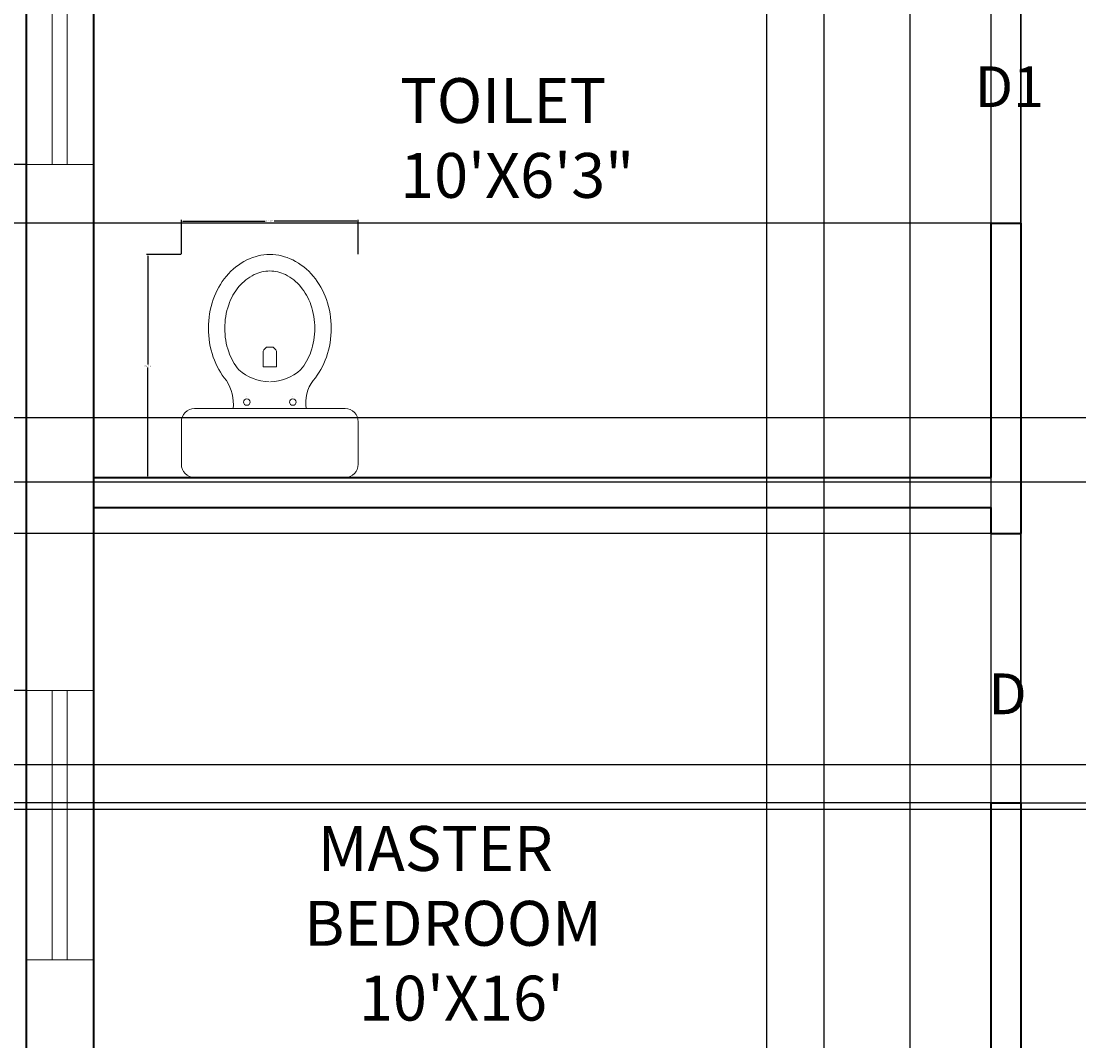
# Model space of a CAD drawing. Units: inches. Extents: x 503 to 1084, y -605 to 132.
# Tile 5 of 14: x 649 to 791, y -313 to -177. Entities that reach past the tile are written whole.
import ezdxf

# ---------------------------------------------------------------- set-up
doc = ezdxf.new("R2010")
doc.units = ezdxf.units.IN
doc.header["$MEASUREMENT"] = 0
for name, color, linetype, lineweight in [('A-ANNO-DIMS', 7, 'Continuous', 18), ('A-ANNO-TEXT', 7, 'Continuous', 18), ('A-AREA-IDEN', 8, 'Continuous', 18), ('A-FLOR-FIXT', 8, 'Continuous', 18), ('wall', 1, 'Continuous', 35), ('wind', 5, 'Continuous', 18)]:
    doc.layers.add(name, color=color, linetype=linetype, lineweight=lineweight)
doc.styles.get("Standard").update_dxf_attribs({"font": 'arial.ttf'})
doc.dimstyles.get("Standard").update_dxf_attribs({"dimtxt": 0.18, "dimasz": 0.18, "dimexe": 0.18, "dimexo": 0.0625, "dimgap": 0.09, "dimtad": 0, "dimtih": 1, "dimtoh": 1, "dimdec": 1, "dimzin": 0, "dimdsep": 46, "dimlunit": 4, "dimtxsty": 'Standard', "dimcen": 0.09, "dimadec": 0, "dimazin": 0, "dimtfac": 1, "dimtdec": 1, "dimtofl": 0, "dimtmove": 0, "dimatfit": 3, "dimfxl": 1, "dimtolj": 1, "dimtzin": 0, "dimarcsym": 0})

# ---------------------------------------------------------------- blocks, each defined once
blk = doc.blocks.new('WC-P01')
for p, q in [((-230, 0), (230, 0)), ((-270, -40), (-270, -170)), ((270, -40), (270, -170)), ((-230, -210), (230, -210)), ((-111.4, -210), (-111.4, -210)), ((-20, -337.8), (20, -337.8)), ((-20, -337.8), (-20, -385.7)), ((20, -337.8), (20, -385.7)), ((-18.5, -389.3), (-10.5, -397.3)), ((-10.5, -397.3), (10.5, -397.3)), ((10.5, -397.3), (18.5, -389.3))]:
    blk.add_line(p, q)
for points in [[(-111.4, -210, -0.215497), (-132.6, -295.9, 0.09084), (-172.8, -367.1, 0.083285), (-187.5, -455, 0.083285), (-172.8, -542.9, 0.09084), (-132.6, -614.1, 0.104065), (-70, -663.6, 0.115836), (0, -680, 0.115836), (70, -663.6, 0.104065), (132.6, -614.1, 0.09084), (172.8, -542.9, 0.083285), (187.5, -455, 0.083285)], [(187.5, -455, 0.083285), (172.8, -367.1, 0.09084), (132.6, -295.9, -0.156524), (111.4, -210)], [(-70, -246.4), (-70, -246.4, 0.104065)], [(70, -246.4), (70, -246.4, 0.115836)], [(-1.8, -291.3, 0.171753), (-94.2, -327.9, 0.09084), (-125.5, -383.5, 0.083285), (-137.5, -455, 0.083285), (-125.5, -526.5, 0.09084), (-94.2, -582.1, 0.104065), (-47.7, -618.8, 0.115836), (0, -630, 0.115836)], [(1.8, -291.3, -0.171753), (94.2, -327.9, -0.09084), (125.5, -383.5, -0.083285), (137.5, -455, -0.083285), (125.5, -526.5, -0.09084), (94.2, -582.1, -0.104065), (47.7, -618.8, -0.115836), (0, -630, -0.115836)]]:
    blk.add_lwpolyline(points, format="xyb")
for centre in [(-70, -230), (70, -230)]:
    blk.add_circle(centre, 10)
for centre, radius, start, end in [((-230, -40), 40, 90, 180), ((230, -40), 40, 0, 90), ((-230, -170), 40, 180, 270), ((230, -170), 40, 270, 0), ((-15, -385.7), 5, 180, 225), ((15, -385.7), 5, 315, 0)]:
    blk.add_arc(centre, radius, start, end)
blk = doc.blocks.new('_ArchTick')
at = {"color": 0, "linetype": 'ByBlock', "const_width": 0.15}
blk.add_lwpolyline([(-0.5, -0.5), (0.5, 0.5)], dxfattribs=at)
blk = doc.blocks.new('_Oblique')
at = {"color": 0, "linetype": 'ByBlock', "lineweight": -2}
blk.add_line((-0.5, -0.5), (0.5, 0.5), dxfattribs=at)
blk = doc.blocks.new('*D12')
at = {"layer": 'A-ANNO-DIMS', "color": 0, "lineweight": -2, "transparency": 16777216}
blk.add_line((554.79, -17.82), (554.79, -442.82), dxfattribs=at)
at = {"layer": 'Defpoints', "color": 0, "transparency": 16777216}
for p in [(650.09, -17.82), (554.79, -442.82), (650.09, -442.82)]:
    blk.add_point(p, dxfattribs=at)
at = {"layer": 'A-ANNO-DIMS', "color": 0, "lineweight": -2, "transparency": 16777216, "xscale": 5, "yscale": 5, "zscale": 5}
for name, p, rotation in [('_ArchTick', (554.79, -17.82), 90), ('_Oblique', (554.79, -442.82), 270)]:
    blk.add_blockref(name, p, dxfattribs=dict(at, rotation=rotation))
at = {"layer": 'A-ANNO-DIMS', "color": 0, "transparency": 16777216, "insert": (546.7, -230.32), "char_height": 8, "attachment_point": 5, "rotation": 90}
blk.add_mtext("\\A1;36'", dxfattribs=at)
blk = doc.blocks.new('WIN-36IN')
for p, q in [((0, 0), (0, 9)), ((36, 0), (36, 9)), ((0, 5.5), (36, 5.5)), ((0, 3.5), (36, 3.5))]:
    blk.add_line(p, q)
blk = doc.blocks.new('VENT-24IN')
for p, q in [((0, 9), (0, 0)), ((24, 9), (24, 0)), ((24, 5.5), (0, 5.5)), ((24, 3.5), (0, 3.5))]:
    blk.add_line(p, q)
blk = doc.blocks.new('*D32')
at = {"layer": 'A-ANNO-DIMS', "color": 0, "lineweight": -2, "transparency": 16777216}
for p, q in [((670.79, -208.03), (666.21, -208.03)), ((666.39, -208.21), (666.39, -222.74)), ((666.39, -237.64), (666.39, -223.11)), ((670.79, -237.82), (666.21, -237.82))]:
    blk.add_line(p, q, dxfattribs=at)
at = {"layer": 'A-ANNO-DIMS', "color": 0, "transparency": 16777216}
for points in [[(666.36, -208.21), (666.42, -208.21), (666.39, -208.03)], [(666.36, -237.64), (666.42, -237.64), (666.39, -237.82)]]:
    blk.add_solid(points, dxfattribs=at)
at = {"layer": 'Defpoints', "color": 0, "transparency": 16777216}
for p in [(670.86, -208.03), (666.39, -237.82), (670.86, -237.82)]:
    blk.add_point(p, dxfattribs=at)
at = {"layer": 'A-ANNO-DIMS', "color": 0, "transparency": 16777216, "insert": (666.39, -222.92), "char_height": 0.18, "attachment_point": 5}
blk.add_mtext('\\A1;WC 2\'-6"', dxfattribs=at)
blk = doc.blocks.new('*D33')
at = {"layer": 'A-ANNO-DIMS', "color": 0, "lineweight": -2, "transparency": 16777216}
for p, q in [((670.86, -207.97), (670.86, -203.38)), ((671.04, -203.56), (682.08, -203.56)), ((694.33, -203.56), (683.28, -203.56)), ((694.51, -207.97), (694.51, -203.38))]:
    blk.add_line(p, q, dxfattribs=at)
at = {"layer": 'A-ANNO-DIMS', "color": 0, "transparency": 16777216}
for points in [[(671.04, -203.53), (671.04, -203.59), (670.86, -203.56)], [(694.33, -203.53), (694.33, -203.59), (694.51, -203.56)]]:
    blk.add_solid(points, dxfattribs=at)
at = {"layer": 'Defpoints', "color": 0, "transparency": 16777216}
for p in [(670.86, -203.56), (670.86, -208.03), (694.51, -208.03)]:
    blk.add_point(p, dxfattribs=at)
at = {"layer": 'A-ANNO-DIMS', "color": 0, "transparency": 16777216, "insert": (682.68, -203.56), "char_height": 0.18, "attachment_point": 5}
blk.add_mtext('\\A1;1\'-11 1/2"', dxfattribs=at)
blk = doc.blocks.new('*D48')
at = {"layer": 'A-ANNO-DIMS', "color": 0, "lineweight": -2, "transparency": 16777216}
for p, q in [((783.09, -354.75), (783.09, 43.51)), ((783.27, 43.33), (789.22, 43.33)), ((795.82, 43.33), (789.86, 43.33)), ((796, -354.75), (796, 43.51))]:
    blk.add_line(p, q, dxfattribs=at)
at = {"layer": 'A-ANNO-DIMS', "color": 0, "transparency": 16777216}
for points in [[(783.27, 43.36), (783.27, 43.3), (783.09, 43.33)], [(795.82, 43.36), (795.82, 43.3), (796, 43.33)]]:
    blk.add_solid(points, dxfattribs=at)
at = {"layer": 'Defpoints', "color": 0, "transparency": 16777216}
for p in [(796, 43.33), (783.09, -354.82), (796, -354.82)]:
    blk.add_point(p, dxfattribs=at)
at = {"layer": 'A-ANNO-DIMS', "color": 0, "transparency": 16777216, "insert": (789.54, 43.33), "char_height": 0.18, "attachment_point": 5}
blk.add_mtext('\\A1;1\'-1"', dxfattribs=at)
blk = doc.blocks.new('*D54')
at = {"layer": 'A-ANNO-DIMS', "color": 0, "lineweight": -2, "transparency": 16777216}
for p, q in [((650.03, -195.98), (552.76, -195.98)), ((552.94, -196.16), (552.94, -230.97)), ((552.94, -266.14), (552.94, -231.33)), ((650.03, -266.32), (552.76, -266.32))]:
    blk.add_line(p, q, dxfattribs=at)
at = {"layer": 'A-ANNO-DIMS', "color": 0, "transparency": 16777216}
for points in [[(552.91, -196.16), (552.97, -196.16), (552.94, -195.98)], [(552.91, -266.14), (552.97, -266.14), (552.94, -266.32)]]:
    blk.add_solid(points, dxfattribs=at)
at = {"layer": 'Defpoints', "color": 0, "transparency": 16777216}
for p in [(650.09, -195.98), (552.94, -266.32), (650.09, -266.32)]:
    blk.add_point(p, dxfattribs=at)
at = {"layer": 'A-ANNO-DIMS', "color": 0, "transparency": 16777216, "insert": (552.94, -231.15), "char_height": 0.18, "attachment_point": 5}
blk.add_mtext('\\A1;5\'-10 1/2"', dxfattribs=at)
blk = doc.blocks.new('*D55')
at = {"layer": 'A-ANNO-DIMS', "color": 0, "lineweight": -2, "transparency": 16777216}
for p, q in [((779.03, -245.32), (552.76, -245.32)), ((552.94, -245.5), (552.94, -263.13)), ((552.94, -281.14), (552.94, -263.5)), ((779.03, -281.32), (552.76, -281.32))]:
    blk.add_line(p, q, dxfattribs=at)
at = {"layer": 'A-ANNO-DIMS', "color": 0, "transparency": 16777216}
for points in [[(552.91, -245.5), (552.97, -245.5), (552.94, -245.32)], [(552.91, -281.14), (552.97, -281.14), (552.94, -281.32)]]:
    blk.add_solid(points, dxfattribs=at)
at = {"layer": 'Defpoints', "color": 0, "transparency": 16777216}
for p in [(779.09, -245.32), (552.94, -281.32), (779.09, -281.32)]:
    blk.add_point(p, dxfattribs=at)
at = {"layer": 'A-ANNO-DIMS', "color": 0, "transparency": 16777216, "insert": (552.94, -263.32), "char_height": 0.18, "attachment_point": 5}
blk.add_mtext('\\A1;3\'-0"', dxfattribs=at)
blk = doc.blocks.new('*D56')
at = {"layer": 'A-ANNO-DIMS', "color": 0, "lineweight": -2, "transparency": 16777216}
for p, q in [((779.03, -167.82), (552.76, -167.82)), ((552.94, -168), (552.94, -185.63)), ((552.94, -203.64), (552.94, -186)), ((779.03, -203.82), (552.76, -203.82))]:
    blk.add_line(p, q, dxfattribs=at)
at = {"layer": 'A-ANNO-DIMS', "color": 0, "transparency": 16777216}
for points in [[(552.91, -168), (552.97, -168), (552.94, -167.82)], [(552.91, -203.64), (552.97, -203.64), (552.94, -203.82)]]:
    blk.add_solid(points, dxfattribs=at)
at = {"layer": 'Defpoints', "color": 0, "transparency": 16777216}
for p in [(779.09, -167.82), (552.94, -203.82), (779.09, -203.82)]:
    blk.add_point(p, dxfattribs=at)
at = {"layer": 'A-ANNO-DIMS', "color": 0, "transparency": 16777216, "insert": (552.94, -185.82), "char_height": 0.18, "attachment_point": 5}
blk.add_mtext('\\A1;3\'-0"', dxfattribs=at)
blk = doc.blocks.new('*D60')
at = {"layer": 'A-ANNO-DIMS', "color": 0, "lineweight": -2, "transparency": 16777216}
for p, q in [((749.09, -117.88), (749.09, -583.15)), ((779.09, -117.88), (779.09, -583.15)), ((749.27, -582.97), (763.76, -582.97)), ((778.91, -582.97), (764.42, -582.97))]:
    blk.add_line(p, q, dxfattribs=at)
at = {"layer": 'A-ANNO-DIMS', "color": 0, "transparency": 16777216}
for points in [[(749.27, -582.94), (749.27, -583), (749.09, -582.97)], [(778.91, -582.94), (778.91, -583), (779.09, -582.97)]]:
    blk.add_solid(points, dxfattribs=at)
at = {"layer": 'Defpoints', "color": 0, "transparency": 16777216}
for p in [(749.09, -117.82), (779.09, -117.82), (779.09, -582.97)]:
    blk.add_point(p, dxfattribs=at)
at = {"layer": 'A-ANNO-DIMS', "color": 0, "transparency": 16777216, "insert": (764.09, -582.97), "char_height": 0.18, "attachment_point": 5}
blk.add_mtext('\\A1;2\'-6"', dxfattribs=at)
blk = doc.blocks.new('*D62')
at = {"layer": 'A-ANNO-DIMS', "color": 0, "lineweight": -2, "transparency": 16777216}
for p, q in [((779.03, -203.82), (552.76, -203.82)), ((552.94, -204), (552.94, -224.38)), ((552.94, -245.14), (552.94, -224.75)), ((779.03, -245.32), (552.76, -245.32))]:
    blk.add_line(p, q, dxfattribs=at)
at = {"layer": 'A-ANNO-DIMS', "color": 0, "transparency": 16777216}
for points in [[(552.91, -204), (552.97, -204), (552.94, -203.82)], [(552.91, -245.14), (552.97, -245.14), (552.94, -245.32)]]:
    blk.add_solid(points, dxfattribs=at)
at = {"layer": 'Defpoints', "color": 0, "transparency": 16777216}
for p in [(779.09, -203.82), (552.94, -245.32), (779.09, -245.32)]:
    blk.add_point(p, dxfattribs=at)
at = {"layer": 'A-ANNO-DIMS', "color": 0, "transparency": 16777216, "insert": (552.94, -224.57), "char_height": 0.18, "attachment_point": 5}
blk.add_mtext('\\A1;3\'-5 1/2"', dxfattribs=at)
blk = doc.blocks.new('*D63')
at = {"layer": 'A-ANNO-DIMS', "color": 0, "lineweight": -2, "transparency": 16777216}
for p, q in [((783.15, -281.32), (1083.42, -281.32)), ((1083.24, -281.5), (1083.24, -317.88)), ((1083.24, -354.64), (1083.24, -318.25)), ((783.15, -354.82), (1083.42, -354.82))]:
    blk.add_line(p, q, dxfattribs=at)
at = {"layer": 'A-ANNO-DIMS', "color": 0, "transparency": 16777216}
for points in [[(1083.21, -281.5), (1083.27, -281.5), (1083.24, -281.32)], [(1083.21, -354.64), (1083.27, -354.64), (1083.24, -354.82)]]:
    blk.add_solid(points, dxfattribs=at)
at = {"layer": 'Defpoints', "color": 0, "transparency": 16777216}
for p in [(783.09, -281.32), (783.09, -354.82), (1083.24, -354.82)]:
    blk.add_point(p, dxfattribs=at)
at = {"layer": 'A-ANNO-DIMS', "color": 0, "transparency": 16777216, "insert": (1083.24, -318.07), "char_height": 0.18, "attachment_point": 5}
blk.add_mtext('\\A1;6\'-1 1/2"', dxfattribs=at)
blk = doc.blocks.new('*D68')
at = {"layer": 'A-ANNO-DIMS', "color": 0, "lineweight": -2, "transparency": 16777216}
for p, q in [((779.09, -117.88), (779.09, -583.15)), ((783.09, -117.88), (783.09, -583.15)), ((779.27, -582.97), (780.76, -582.97)), ((782.91, -582.97), (781.42, -582.97))]:
    blk.add_line(p, q, dxfattribs=at)
at = {"layer": 'A-ANNO-DIMS', "color": 0, "transparency": 16777216}
for points in [[(779.27, -582.94), (779.27, -583), (779.09, -582.97)], [(782.91, -582.94), (782.91, -583), (783.09, -582.97)]]:
    blk.add_solid(points, dxfattribs=at)
at = {"layer": 'Defpoints', "color": 0, "transparency": 16777216}
for p in [(779.09, -117.82), (783.09, -117.82), (783.09, -582.97)]:
    blk.add_point(p, dxfattribs=at)
at = {"layer": 'A-ANNO-DIMS', "color": 0, "transparency": 16777216, "insert": (781.09, -582.97), "char_height": 0.18, "attachment_point": 5}
blk.add_mtext('\\A1;0\'-4"', dxfattribs=at)
blk = doc.blocks.new('*D72')
at = {"layer": 'A-ANNO-DIMS', "color": 0, "lineweight": -2, "transparency": 16777216}
for p, q in [((948.89, -229.87), (552.76, -229.87)), ((552.94, -230.05), (552.94, -255.86)), ((552.94, -282.03), (552.94, -256.22)), ((949.25, -282.21), (552.76, -282.21))]:
    blk.add_line(p, q, dxfattribs=at)
at = {"layer": 'A-ANNO-DIMS', "color": 0, "transparency": 16777216}
for points in [[(552.91, -230.05), (552.97, -230.05), (552.94, -229.87)], [(552.91, -282.03), (552.97, -282.03), (552.94, -282.21)]]:
    blk.add_solid(points, dxfattribs=at)
at = {"layer": 'Defpoints', "color": 0, "transparency": 16777216}
for p in [(948.95, -229.87), (552.94, -282.21), (949.31, -282.21)]:
    blk.add_point(p, dxfattribs=at)
at = {"layer": 'A-ANNO-DIMS', "color": 0, "transparency": 16777216, "insert": (552.94, -256.04), "char_height": 0.18, "attachment_point": 5}
blk.add_mtext('\\A1;4\'-4 1/2"', dxfattribs=at)
blk = doc.blocks.new('*D76')
at = {"layer": 'A-ANNO-DIMS', "color": 0, "lineweight": -2, "transparency": 16777216}
for p, q in [((756.77, -45.47), (756.77, -583.15)), ((768.24, -45.47), (768.24, -583.15)), ((756.95, -582.97), (761.9, -582.97)), ((768.06, -582.97), (763.11, -582.97))]:
    blk.add_line(p, q, dxfattribs=at)
at = {"layer": 'A-ANNO-DIMS', "color": 0, "transparency": 16777216}
for points in [[(756.95, -582.94), (756.95, -583), (756.77, -582.97)], [(768.06, -582.94), (768.06, -583), (768.24, -582.97)]]:
    blk.add_solid(points, dxfattribs=at)
at = {"layer": 'Defpoints', "color": 0, "transparency": 16777216}
for p in [(756.77, -45.4), (768.24, -45.4), (768.24, -582.97)]:
    blk.add_point(p, dxfattribs=at)
at = {"layer": 'A-ANNO-DIMS', "color": 0, "transparency": 16777216, "insert": (762.51, -582.97), "char_height": 0.18, "attachment_point": 5}
blk.add_mtext('\\A1;0\'-11 1/2"', dxfattribs=at)
blk = doc.blocks.new('*D77')
at = {"layer": 'A-ANNO-DIMS', "color": 0, "lineweight": -2, "transparency": 16777216}
for p, q in [((926.53, -238.47), (552.76, -238.47)), ((552.94, -238.65), (552.94, -257.17)), ((552.94, -276.07), (552.94, -257.54)), ((916.28, -276.25), (552.76, -276.25))]:
    blk.add_line(p, q, dxfattribs=at)
at = {"layer": 'A-ANNO-DIMS', "color": 0, "transparency": 16777216}
for points in [[(552.91, -238.65), (552.97, -238.65), (552.94, -238.47)], [(552.91, -276.07), (552.97, -276.07), (552.94, -276.25)]]:
    blk.add_solid(points, dxfattribs=at)
at = {"layer": 'Defpoints', "color": 0, "transparency": 16777216}
for p in [(926.59, -238.47), (552.94, -276.25), (916.35, -276.25)]:
    blk.add_point(p, dxfattribs=at)
at = {"layer": 'A-ANNO-DIMS', "color": 0, "transparency": 16777216, "insert": (552.94, -257.36), "char_height": 0.18, "attachment_point": 5}
blk.add_mtext('\\A1;3\'-2"', dxfattribs=at)

msp = doc.modelspace()

# ---------------------------------------------------------------- linework, layer by layer
at = {"layer": 'wall'}
for p, q in [((650.09, -17.82), (650.09, -514.82)), ((659.09, -26.82), (659.09, -433.82)), ((779.09, -203.82), (783.09, -203.82)), ((779.09, -203.82), (779.09, -237.82)), ((783.09, -203.82), (783.09, -245.32)), ((659.09, -237.82), (779.09, -237.82)), ((659.09, -241.82), (779.09, -241.82)), ((779.09, -241.82), (779.09, -245.32)), ((779.09, -245.32), (783.09, -245.32)), ((779.09, -281.32), (783.09, -281.32)), ((779.09, -281.32), (779.09, -433.82)), ((783.09, -281.32), (783.09, -354.82))]:
    msp.add_line(p, q, dxfattribs=at)

# ---------------------------------------------------------------- block references
at = {"layer": 'A-FLOR-FIXT', "xscale": 0.0438047028060103, "yscale": 0.0438047028060103, "zscale": 0.0438047028060103, "rotation": 180}
msp.add_blockref('WC-P01', (682.68, -237.82), dxfattribs=at)
at = {"layer": 'wind'}
for name, p, rotation in [('VENT-24IN', (659.09, -195.98), 90.00000000000081), ('WIN-36IN', (659.09, -302.31), 90.00000000000033)]:
    msp.add_blockref(name, p, dxfattribs=dict(at, rotation=rotation))

# ---------------------------------------------------------------- texts
at = {"layer": 'A-ANNO-TEXT'}
for s, height, p in [('D1', 5.444, (776.95, -188.32)), ('D', 5.44, (778.77, -269.47))]:
    msp.add_text(s, height=height, dxfattribs=at).set_placement(p)
at = {"layer": 'A-AREA-IDEN', "char_height": 6, "attachment_point": 1}
for s, width, insert in [('       TOILET\\P       10\'X6\'3"', 54.3765, (687.27, -184.45)), (" MASTER BEDROOM\\P    10'X16'", 45.6749, (687.27, -284.42))]:
    msp.add_mtext_dynamic_manual_height_columns(s, width=width, gutter_width=1, heights=[0], dxfattribs=dict(at, insert=insert))

# ---------------------------------------------------------------- dimensions: what is measured, and where the dimension line sits
at = {"layer": 'A-ANNO-DIMS'}
for base, p1, p2, picture, middle in [((796, 43.33), (783.09, -354.82), (796, -354.82), '*D48', (789.54, 43.33)), ((768.24, -582.97), (756.77, -45.4), (768.24, -45.4), '*D76', (762.51, -582.97)), ((779.09, -582.97), (749.09, -117.82), (779.09, -117.82), '*D60', (764.09, -582.97)), ((783.09, -582.97), (779.09, -117.82), (783.09, -117.82), '*D68', (781.09, -582.97))]:
    dim = msp.add_linear_dim(base=base, p1=p1, p2=p2, dimstyle='Standard', override={"dimdec": 1, "dimlfac": 1, "dimrnd": 0, "dimzin": 1, "dimdsep": 46, "dimlunit": 4, "dimfrac": 2}, dxfattribs=at)
    dim.commit()
    dim.dimension.update_dxf_attribs({"geometry": picture, "text_midpoint": middle})
for base, p1, p2, angle, text, override, picture, middle in [((554.79, -442.82), (650.09, -17.82), (650.09, -442.82), 90, "36'", {"dimtxt": 8, "dimasz": 5, "dimgap": 4, "dimtad": 1, "dimtih": 0, "dimblk1": 'ArchTick', "dimblk2": 'Oblique', "dimsah": 1, "dimse1": 1, "dimse2": 1, "dimclrd": 0, "dimclre": 0, "dimclrt": 0}, '*D12', (546.7, -230.32)), ((666.39, -237.82), (670.86, -208.03), (670.86, -237.82), 270, 'WC <>', {"dimdec": 1, "dimlfac": 1, "dimrnd": 0, "dimzin": 1, "dimdsep": 46, "dimlunit": 4, "dimfrac": 2}, '*D32', (666.39, -222.92))]:
    dim = msp.add_linear_dim(base=base, p1=p1, p2=p2, angle=angle, text=text, dimstyle='Standard', override=override, dxfattribs=at)
    dim.commit()
    dim.dimension.update_dxf_attribs({"geometry": picture, "text_midpoint": middle})
for base, p1, p2, angle, picture, middle in [((552.94, -203.82), (779.09, -167.82), (779.09, -203.82), 90, '*D56', (552.94, -185.82)), ((552.94, -266.32), (650.09, -195.98), (650.09, -266.32), 90, '*D54', (552.94, -231.15)), ((670.8553, -203.5606), (694.5099, -208.0287), (670.8553, -208.0287), 180, '*D33', (682.6826, -203.5606)), ((552.94, -245.32), (779.09, -203.82), (779.09, -245.32), 90, '*D62', (552.94, -224.57)), ((552.94, -282.21), (948.95, -229.87), (949.31, -282.21), 90, '*D72', (552.94, -256.04)), ((552.94, -276.25), (926.59, -238.47), (916.35, -276.25), 90, '*D77', (552.94, -257.36)), ((552.94, -281.32), (779.09, -245.32), (779.09, -281.32), 90, '*D55', (552.94, -263.32)), ((1083.24, -354.82), (783.09, -281.32), (783.09, -354.82), 90, '*D63', (1083.24, -318.07))]:
    dim = msp.add_linear_dim(base=base, p1=p1, p2=p2, angle=angle, dimstyle='Standard', override={"dimdec": 1, "dimlfac": 1, "dimrnd": 0, "dimzin": 1, "dimdsep": 46, "dimlunit": 4, "dimfrac": 2}, dxfattribs=at)
    dim.commit()
    dim.dimension.update_dxf_attribs({"geometry": picture, "text_midpoint": middle})

doc.saveas('drawing.dxf')
